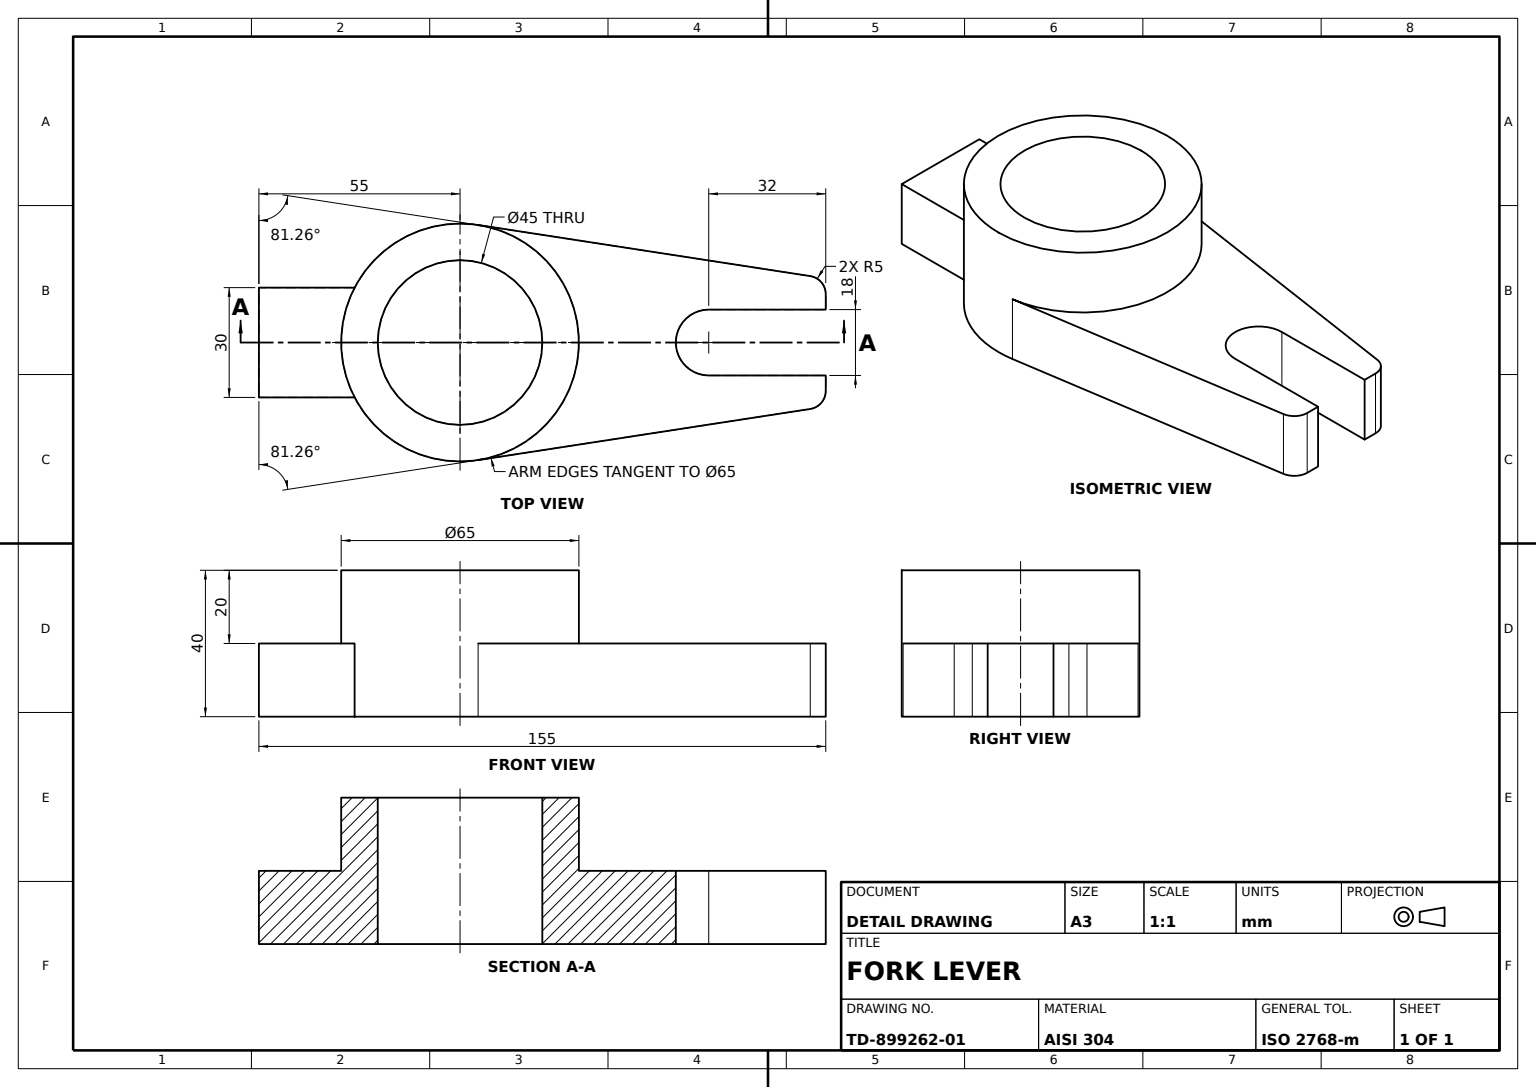
SolidWorks part; units mm, degrees
material "AISI 304"
ref_plane "Front Plane" through (0, 0, 0) normal (0, 0, 1) x (1, 0, 0)
ref_plane "Top Plane" through (0, 0, 0) normal (0, 1, 0) x (1, 0, 0)
ref_plane "Right Plane" through (0, 0, 0) normal (1, 0, 0) x (0, 0, -1)
sketch "Hub Ring Sketch" plane through (0, 0, 0) normal (0, 1, 0) x (1, 0, 0)
  circle A0 centre (0, 0) radius 32.5
  circle A1 centre (0, 0) radius 22.5
  dimension "D1" = 65
  dimension "D2" = 45
extrude "Hub Ring Ø65xØ45" add sketch "Hub Ring Sketch" along normal mid plane 40
sketch "Fork Arm Sketch" plane through (0, 0, 0) normal (0, 1, 0) x (1, 0, 0)
  line L0 (95.7602, 18.1522) -> (4.9411, 32.1222)
  line L1 (100, 13.2103) -> (100, 9)
  line L2 (100, 9) -> (68, 9)
  line L3 (68, -9) -> (100, -9)
  line L4 (100, -9) -> (100, -13.2103)
  line L5 (95.7602, -18.1522) -> (4.9411, -32.1222)
  circle A0 centre (0, 0) radius 32.5 construction
  arc A1 (68, 9) -> (68, -9) centre (68, 0) ccw
  arc A2 (100, -13.2103) -> (95.7602, -18.1522) centre (95, -13.2103) cw
  arc A3 (95.7602, 18.1522) -> (100, 13.2103) centre (95, 13.2103) cw
  arc A4 (4.9411, -32.1222) -> (4.9411, 32.1222) centre (0, 0) ccw
  point P12 (100, -17.5)
  point P16 (100, 17.5)
  dimension "D3" = 5
  dimension "D1" = 32
  dimension "D2" = 35
  dimension "D4" = 100
  dimension "D5" = 18
extrude "Fork Arm" add sketch "Fork Arm Sketch" against normal blind 20
sketch "Rear Tab Sketch" plane through (0, 0, 0) normal (0, 1, 0) x (1, 0, 0)
  line L0 (-28.8314, 15) -> (-55, 15)
  line L1 (-55, 15) -> (-55, -15)
  line L2 (-55, -15) -> (-28.8314, -15)
  circle A0 centre (0, 0) radius 32.5 construction
  arc A1 (-28.8314, 15) -> (-28.8314, -15) centre (0, 0) ccw
  point P7 (-55, 0)
  dimension "D1" = 30
  dimension "D2" = 55
extrude "Rear Tab" add sketch "Rear Tab Sketch" against normal blind 20
